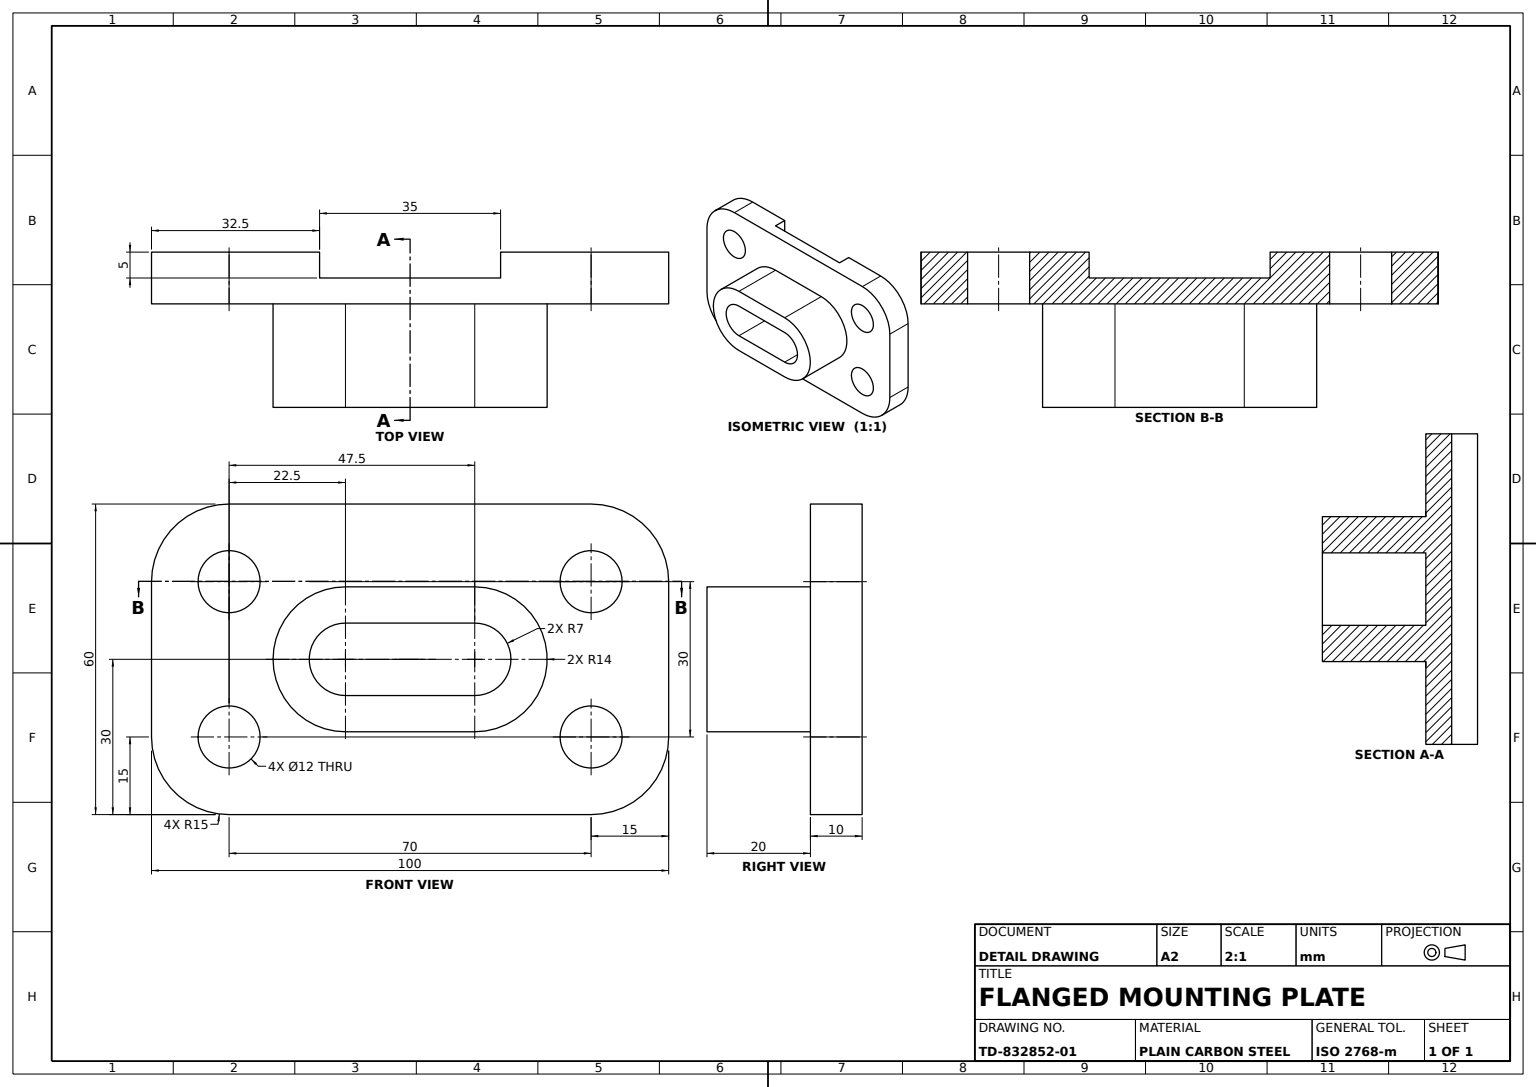
from build123d import *

# Parameters (mm, degrees)
BASE_PLATE_DEPTH        = 10
MOUNTING_HOLES_SKETCH_R = 6
MOUNTING_HOLES_4X_DEPTH = 10
SLOT_BOSS_DEPTH         = 20
SLOT_THROUGH_CUT_DEPTH  = 20
BACK_CHANNEL_CUT_DEPTH  = 60


with BuildPart() as part:
    # Base Plate Sketch → Base Plate (new body)
    with BuildSketch(Plane.XY):
        with BuildLine():
            Line((15, 0), (85, 0))
            ThreePointArc((85, 0), (95.606601718, -4.393398282), (100, -15))
            Line((100, -15), (100, -45))
            ThreePointArc((100, -45), (95.606601718, -55.606601718), (85, -60))
            Line((85, -60), (15, -60))
            ThreePointArc((15, -60), (4.393398282, -55.606601718), (0, -45))
            Line((0, -45), (0, -15))
            ThreePointArc((0, -15), (4.393398282, -4.393398282), (15, 0))
        make_face()
    extrude(amount=BASE_PLATE_DEPTH)

    # Mounting Holes Sketch → Mounting Holes 4x (cut)
    with BuildSketch(Plane.XY.offset(10)):
        with Locations((15, -15)):
            Circle(MOUNTING_HOLES_SKETCH_R)
        with Locations((85, -15)):
            Circle(MOUNTING_HOLES_SKETCH_R)
        with Locations((85, -45)):
            Circle(MOUNTING_HOLES_SKETCH_R)
        with Locations((15, -45)):
            Circle(MOUNTING_HOLES_SKETCH_R)
    extrude(amount=-MOUNTING_HOLES_4X_DEPTH, mode=Mode.SUBTRACT)

    # Slot Boss Sketch → Slot Boss (add)
    with BuildSketch(Plane.XY.offset(10)):
        with BuildLine():
            Line((37.5, -16), (62.5, -16))
            ThreePointArc((62.5, -16), (76.5, -30), (62.5, -44))
            Line((62.5, -44), (37.5, -44))
            ThreePointArc((37.5, -44), (23.5, -30), (37.5, -16))
        make_face()
    extrude(amount=SLOT_BOSS_DEPTH)

    # Slot Cut Sketch → Slot Through Cut (cut)
    with BuildSketch(Plane.XY.offset(30)):
        with BuildLine():
            Line((37.5, -23), (62.5, -23))
            ThreePointArc((62.5, -23), (69.5, -30), (62.5, -37))
            Line((62.5, -37), (37.5, -37))
            ThreePointArc((37.5, -37), (30.5, -30), (37.5, -23))
        make_face()
    extrude(amount=-SLOT_THROUGH_CUT_DEPTH, mode=Mode.SUBTRACT)

    # Back Channel Sketch → Back Channel Cut (cut)
    with BuildSketch(Plane.XZ.offset(60)):
        Polygon((50, 0), (67.5, 0), (67.5, 5), (32.5, 5), (32.5, 0), align=None)
    extrude(amount=-BACK_CHANNEL_CUT_DEPTH, mode=Mode.SUBTRACT)


solid = part.part
